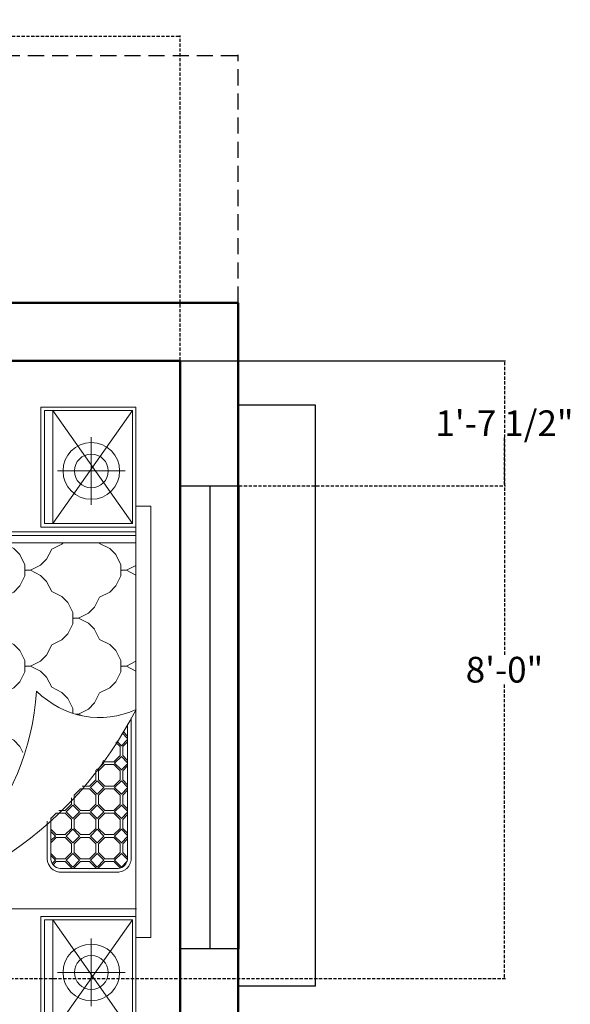
# Model space of a CAD drawing. Units: inches. Extents: x 513 to 1142, y 396 to 927.
# Tile 31 of 31: x 1056 to 1142, y 770 to 923. Entities that reach past the tile are written whole.
import ezdxf

# ---------------------------------------------------------------- set-up
doc = ezdxf.new("R2010")
doc.units = ezdxf.units.IN
doc.header["$MEASUREMENT"] = 0
doc.linetypes.add('DASHED', pattern=[0.75, 0.5, -0.25])
for name, color, linetype, lineweight in [('A-ANNO-DIMS', 2, 'DASHED', 18), ('A-WALL', 7, 'Continuous', 50), ('furniture', 92, 'Continuous', 18), ('windows', 172, 'Continuous', 25)]:
    doc.layers.add(name, color=color, linetype=linetype, lineweight=lineweight)
doc.styles.get("Standard").update_dxf_attribs({"font": 'arial.ttf'})
doc.dimstyles.get("Standard").update_dxf_attribs({"dimtxt": 4, "dimasz": 0.18, "dimexe": 0.18, "dimexo": 0.0625, "dimgap": 0.09, "dimtad": 0, "dimtih": 1, "dimtoh": 1, "dimdec": 0, "dimrnd": 6, "dimzin": 0, "dimdsep": 46, "dimlunit": 3, "dimtxsty": 'Standard', "dimcen": 0.09, "dimadec": 0, "dimazin": 0, "dimtfac": 1, "dimtdec": 0, "dimtofl": 0, "dimtmove": 0, "dimatfit": 3, "dimfxl": 1, "dimtolj": 1, "dimtzin": 0, "dimarcsym": 0})

# ---------------------------------------------------------------- blocks, each defined once
blk = doc.blocks.new('A$C029D5C69')
for p, q in [((0.4164, 2.0693), (0.4164, 2.0066)), ((2.2315, 2.0693), (0.4164, 2.0693)), ((2.2315, 2.0066), (2.2315, 2.0693)), ((0, 1.606), (0, 2.0066)), ((0, 2.0066), (0.505, 2.0066)), ((0.0151, 1.6211), (0.0151, 1.9915)), ((0.0151, 1.9915), (0.4899, 1.9915)), ((0.4164, 2.0066), (2.2315, 2.0066)), ((0.4899, 1.9915), (0.4899, 1.6211)), ((0.505, 2.0066), (0.505, 1.606)), ((0.5252, 0.0351), (0.5252, 2.0066)), ((0.5403, 0.0502), (0.5403, 2.0066)), ((0.5706, 0.0805), (0.5706, 2.0066)), ((0.6869, 1.966), (0.6666, 2.0066)), ((0.7072, 2.0066), (0.6869, 1.966)), ((1.0902, 1.966), (1.0699, 2.0066)), ((1.1106, 2.0066), (1.0902, 1.966)), ((2.1114, 2.0087), (2.1114, 0.0351)), ((2.6479, 2.0066), (2.1429, 2.0066)), ((2.1429, 2.0066), (2.1429, 1.606)), ((2.6328, 1.9915), (2.158, 1.9915)), ((2.158, 1.9915), (2.158, 1.6211)), ((2.6328, 1.6211), (2.6328, 1.9915)), ((2.6479, 1.606), (2.6479, 2.0066)), ((0.2689, 1.9609), (0.2689, 1.6764)), ((0.6869, 1.9425), (0.6869, 1.966)), ((0.6869, 1.9425), (0.6869, 1.966)), ((1.0902, 1.9425), (1.0902, 1.966)), ((1.0902, 1.9425), (1.0902, 1.966)), ((1.8954, 1.9865), (1.3081, 1.9865)), ((1.8954, 1.9713), (1.3339, 1.9713)), ((1.3849, 1.9713), (1.3656, 1.952)), ((1.3945, 1.9713), (1.3714, 1.9483)), ((1.4249, 1.945), (1.3986, 1.9713)), ((1.4288, 1.9507), (1.4081, 1.9713)), ((1.4476, 1.9507), (1.4288, 1.9507)), ((1.4476, 1.9507), (1.4664, 1.9507)), ((1.487, 1.9713), (1.4664, 1.9507)), ((1.4966, 1.9713), (1.4703, 1.945)), ((1.527, 1.945), (1.5007, 1.9713)), ((1.5309, 1.9507), (1.5102, 1.9713)), ((1.5497, 1.9507), (1.5309, 1.9507)), ((1.5497, 1.9507), (1.5685, 1.9507)), ((1.5891, 1.9713), (1.5685, 1.9507)), ((1.5987, 1.9713), (1.5724, 1.945)), ((1.6291, 1.945), (1.6028, 1.9713)), ((1.633, 1.9507), (1.6123, 1.9713)), ((1.6518, 1.9507), (1.633, 1.9507)), ((1.6518, 1.9507), (1.6706, 1.9507)), ((1.6912, 1.9713), (1.6706, 1.9507)), ((1.7008, 1.9713), (1.6745, 1.945)), ((1.7312, 1.945), (1.7049, 1.9713)), ((1.7351, 1.9507), (1.7144, 1.9713)), ((1.7539, 1.9507), (1.7351, 1.9507)), ((1.7539, 1.9507), (1.7727, 1.9507)), ((1.7933, 1.9713), (1.7727, 1.9507)), ((1.8029, 1.9713), (1.7766, 1.945)), ((1.8333, 1.945), (1.807, 1.9713)), ((1.8372, 1.9507), (1.8165, 1.9713)), ((1.856, 1.9507), (1.8372, 1.9507)), ((1.856, 1.9507), (1.8748, 1.9507)), ((1.8954, 1.9713), (1.8748, 1.9507)), ((1.9043, 1.9707), (1.8787, 1.945)), ((1.9354, 1.945), (1.9114, 1.969)), ((2.379, 1.9609), (2.379, 1.6764)), ((0.621, 1.9213), (0.5955, 1.8958)), ((0.6634, 1.9425), (0.621, 1.9213)), ((0.6634, 1.9425), (0.621, 1.9213)), ((0.6869, 1.9425), (0.6634, 1.9425)), ((0.6869, 1.9425), (0.7104, 1.9425)), ((0.7528, 1.9213), (0.7104, 1.9425)), ((0.7528, 1.9213), (0.7104, 1.9425)), ((0.7783, 1.8958), (0.7528, 1.9213)), ((1.0243, 1.9213), (0.9988, 1.8958)), ((1.0668, 1.9425), (1.0244, 1.9213)), ((1.0668, 1.9425), (1.0244, 1.9213)), ((1.0902, 1.9425), (1.0668, 1.9425)), ((1.0902, 1.9425), (1.1137, 1.9425)), ((1.1561, 1.9213), (1.1137, 1.9425)), ((1.1561, 1.9213), (1.1137, 1.9425)), ((1.1816, 1.8958), (1.1561, 1.9213)), ((1.4249, 1.945), (1.4059, 1.926)), ((1.4288, 1.9394), (1.4116, 1.9222)), ((1.4288, 1.9393), (1.4476, 1.9393)), ((1.4664, 1.9393), (1.4476, 1.9393)), ((1.493, 1.9128), (1.4664, 1.9394)), ((1.4986, 1.9167), (1.4703, 1.945)), ((1.493, 1.8752), (1.493, 1.9128)), ((1.527, 1.945), (1.4986, 1.9167)), ((1.5309, 1.9394), (1.5043, 1.9128)), ((1.5043, 1.8752), (1.5043, 1.9128)), ((1.5309, 1.9393), (1.5497, 1.9393)), ((1.5685, 1.9393), (1.5497, 1.9393)), ((1.595, 1.9128), (1.5685, 1.9394)), ((1.6007, 1.9167), (1.5724, 1.945)), ((1.595, 1.8752), (1.595, 1.9128)), ((1.6291, 1.945), (1.6007, 1.9167)), ((1.633, 1.9394), (1.6064, 1.9128)), ((1.6064, 1.8752), (1.6064, 1.9128)), ((1.633, 1.9393), (1.6518, 1.9393)), ((1.6706, 1.9393), (1.6518, 1.9393)), ((1.6971, 1.9128), (1.6706, 1.9394)), ((1.7028, 1.9167), (1.6745, 1.945)), ((1.6971, 1.8752), (1.6971, 1.9128)), ((1.7312, 1.945), (1.7028, 1.9167)), ((1.7351, 1.9394), (1.7085, 1.9128)), ((1.7085, 1.8752), (1.7085, 1.9128)), ((1.7351, 1.9393), (1.7539, 1.9393)), ((1.7727, 1.9393), (1.7539, 1.9393)), ((1.7992, 1.9128), (1.7727, 1.9394)), ((1.8049, 1.9167), (1.7766, 1.945)), ((1.7992, 1.8752), (1.7992, 1.9128)), ((1.8333, 1.945), (1.8049, 1.9167)), ((1.8372, 1.9394), (1.8106, 1.9128)), ((1.8106, 1.8752), (1.8106, 1.9128)), ((1.8372, 1.9393), (1.856, 1.9393)), ((1.8748, 1.9393), (1.856, 1.9393)), ((1.9013, 1.9128), (1.8748, 1.9394)), ((1.907, 1.9167), (1.8787, 1.945)), ((1.9013, 1.8752), (1.9013, 1.9128)), ((1.9354, 1.945), (1.907, 1.9167)), ((1.9393, 1.9394), (1.9127, 1.9128)), ((1.9127, 1.8752), (1.9127, 1.9128)), ((1.9393, 1.9393), (1.9404, 1.9393)), ((1.9414, 1.688), (1.9414, 1.931)), ((1.9565, 1.688), (1.9565, 1.931)), ((0.5955, 1.8958), (0.5743, 1.8534)), ((0.7995, 1.8534), (0.7783, 1.8958)), ((0.9989, 1.8958), (0.9777, 1.8534)), ((1.2028, 1.8534), (1.1816, 1.8958)), ((1.493, 1.8752), (1.4867, 1.869)), ((1.4986, 1.8713), (1.4922, 1.8648)), ((1.527, 1.8429), (1.4986, 1.8713)), ((1.5309, 1.8486), (1.5043, 1.8752)), ((1.595, 1.8752), (1.5685, 1.8486)), ((1.6007, 1.8713), (1.5724, 1.8429)), ((1.6291, 1.8429), (1.6007, 1.8713)), ((1.633, 1.8486), (1.6064, 1.8752)), ((1.6971, 1.8752), (1.6706, 1.8486)), ((1.7028, 1.8713), (1.6745, 1.8429)), ((1.7312, 1.8429), (1.7028, 1.8713)), ((1.7351, 1.8486), (1.7085, 1.8752)), ((1.7992, 1.8752), (1.7727, 1.8486)), ((1.8049, 1.8713), (1.7766, 1.8429)), ((1.8333, 1.8429), (1.8049, 1.8713)), ((1.8372, 1.8486), (1.8106, 1.8752)), ((1.9013, 1.8752), (1.8748, 1.8486)), ((1.907, 1.8713), (1.8787, 1.8429)), ((1.9354, 1.8429), (1.907, 1.8713)), ((1.9393, 1.8486), (1.9127, 1.8752)), ((0.5743, 1.8534), (0.5706, 1.8515)), ((0.5743, 1.8534), (0.5706, 1.8515)), ((0.8419, 1.8322), (0.7995, 1.8534)), ((0.8419, 1.8322), (0.7995, 1.8534)), ((0.8674, 1.8067), (0.8419, 1.8322)), ((0.9352, 1.8322), (0.9097, 1.8067)), ((0.9777, 1.8534), (0.9353, 1.8322)), ((0.9777, 1.8534), (0.9353, 1.8322)), ((1.2452, 1.8322), (1.2028, 1.8534)), ((1.2452, 1.8322), (1.2028, 1.8534)), ((1.2707, 1.8067), (1.2452, 1.8322)), ((1.527, 1.8429), (1.5242, 1.8401)), ((1.5309, 1.8373), (1.5295, 1.8359)), ((1.5497, 1.8486), (1.5309, 1.8486)), ((1.5309, 1.8373), (1.5497, 1.8373)), ((1.5497, 1.8486), (1.5685, 1.8486)), ((1.5685, 1.8373), (1.5497, 1.8373)), ((1.595, 1.8107), (1.5685, 1.8373)), ((1.6007, 1.8146), (1.5724, 1.8429)), ((1.6291, 1.8429), (1.6007, 1.8146)), ((1.633, 1.8373), (1.6064, 1.8107)), ((1.6518, 1.8486), (1.633, 1.8486)), ((1.633, 1.8373), (1.6518, 1.8373)), ((1.6518, 1.8486), (1.6706, 1.8486)), ((1.6706, 1.8373), (1.6518, 1.8373)), ((1.6971, 1.8107), (1.6706, 1.8373)), ((1.7028, 1.8146), (1.6745, 1.8429)), ((1.7312, 1.8429), (1.7028, 1.8146)), ((1.7351, 1.8373), (1.7085, 1.8107)), ((1.7539, 1.8486), (1.7351, 1.8486)), ((1.7351, 1.8373), (1.7539, 1.8373)), ((1.7539, 1.8486), (1.7727, 1.8486)), ((1.7727, 1.8373), (1.7539, 1.8373)), ((1.7992, 1.8107), (1.7727, 1.8373)), ((1.8049, 1.8146), (1.7766, 1.8429)), ((1.8333, 1.8429), (1.8049, 1.8146)), ((1.8372, 1.8373), (1.8106, 1.8107)), ((1.856, 1.8486), (1.8372, 1.8486)), ((1.8372, 1.8373), (1.856, 1.8373)), ((1.856, 1.8486), (1.8748, 1.8486)), ((1.8748, 1.8373), (1.856, 1.8373)), ((1.9013, 1.8107), (1.8748, 1.8373)), ((1.907, 1.8146), (1.8787, 1.8429)), ((1.9354, 1.8429), (1.907, 1.8146)), ((1.9393, 1.8373), (1.9127, 1.8107)), ((1.9414, 1.8486), (1.9393, 1.8486)), ((1.9393, 1.8373), (1.9414, 1.8373)), ((0.1267, 1.8186), (0.4111, 1.8186)), ((0.8886, 1.7643), (0.8674, 1.8067)), ((0.9098, 1.8067), (0.8886, 1.7643)), ((1.2919, 1.7643), (1.2707, 1.8067)), ((1.595, 1.7806), (1.595, 1.8107)), ((1.6064, 1.7731), (1.6064, 1.8107)), ((1.6971, 1.7731), (1.6971, 1.8107)), ((1.7085, 1.7731), (1.7085, 1.8107)), ((1.7992, 1.7731), (1.7992, 1.8107)), ((1.8106, 1.7731), (1.8106, 1.8107)), ((1.9013, 1.7731), (1.9013, 1.8107)), ((1.9127, 1.7731), (1.9127, 1.8107)), ((2.2367, 1.8186), (2.5212, 1.8186)), ((0.8651, 1.7408), (0.8227, 1.7196)), ((0.8651, 1.7408), (0.8227, 1.7196)), ((0.912, 1.7408), (0.8651, 1.7408)), ((0.8886, 1.7408), (0.8886, 1.7643)), ((0.9544, 1.7196), (0.912, 1.7408)), ((0.9544, 1.7196), (0.912, 1.7408)), ((1.2684, 1.7408), (1.226, 1.7196)), ((1.2684, 1.7408), (1.226, 1.7196)), ((1.2885, 1.7408), (1.2684, 1.7408)), ((1.2981, 1.7768), (1.2919, 1.7643)), ((1.2919, 1.7519), (1.2919, 1.7643)), ((1.633, 1.7465), (1.6064, 1.7731)), ((1.6518, 1.7465), (1.633, 1.7465)), ((1.6518, 1.7465), (1.6706, 1.7465)), ((1.6971, 1.7731), (1.6706, 1.7465)), ((1.7028, 1.7692), (1.6745, 1.7408)), ((1.7028, 1.7125), (1.6745, 1.7408)), ((1.7312, 1.7408), (1.7028, 1.7692)), ((1.7312, 1.7408), (1.7028, 1.7125)), ((1.7351, 1.7465), (1.7085, 1.7731)), ((1.7539, 1.7465), (1.7351, 1.7465)), ((1.7539, 1.7465), (1.7727, 1.7465)), ((1.7992, 1.7731), (1.7727, 1.7465)), ((1.8049, 1.7692), (1.7766, 1.7408)), ((1.8049, 1.7125), (1.7766, 1.7408)), ((1.8333, 1.7408), (1.8049, 1.7692)), ((1.8333, 1.7408), (1.8049, 1.7125)), ((1.8372, 1.7465), (1.8106, 1.7731)), ((1.856, 1.7465), (1.8372, 1.7465)), ((1.856, 1.7465), (1.8748, 1.7465)), ((1.9013, 1.7731), (1.8748, 1.7465)), ((1.907, 1.7692), (1.8787, 1.7408)), ((1.907, 1.7125), (1.8787, 1.7408)), ((1.9354, 1.7408), (1.907, 1.7692)), ((1.9354, 1.7408), (1.907, 1.7125)), ((1.9393, 1.7465), (1.9127, 1.7731)), ((1.9414, 1.7465), (1.9393, 1.7465)), ((0.5766, 1.6941), (0.5706, 1.7002)), ((0.8227, 1.7196), (0.7972, 1.6941)), ((0.98, 1.6941), (0.9545, 1.7196)), ((1.226, 1.7196), (1.2005, 1.6941)), ((1.6443, 1.7352), (1.6518, 1.7352)), ((1.6706, 1.7352), (1.6518, 1.7352)), ((1.6971, 1.7086), (1.6706, 1.7352)), ((1.6971, 1.682), (1.6971, 1.7086)), ((1.7351, 1.7352), (1.7085, 1.7086)), ((1.7085, 1.671), (1.7085, 1.7086)), ((1.7351, 1.7352), (1.7539, 1.7352)), ((1.7727, 1.7352), (1.7539, 1.7352)), ((1.7992, 1.7086), (1.7727, 1.7352)), ((1.7992, 1.671), (1.7992, 1.7086)), ((1.8372, 1.7352), (1.8106, 1.7086)), ((1.8106, 1.671), (1.8106, 1.7086)), ((1.8372, 1.7352), (1.856, 1.7352)), ((1.8748, 1.7352), (1.856, 1.7352)), ((1.9013, 1.7086), (1.8748, 1.7352)), ((1.9013, 1.671), (1.9013, 1.7086)), ((1.9393, 1.7352), (1.9127, 1.7086)), ((1.9127, 1.671), (1.9127, 1.7086)), ((1.9393, 1.7352), (1.9414, 1.7352)), ((0.5978, 1.6517), (0.5766, 1.6941)), ((0.7972, 1.6941), (0.776, 1.6517)), ((1.0011, 1.6517), (0.9799, 1.6941)), ((1.2005, 1.6941), (1.1793, 1.6517)), ((1.7318, 1.6477), (1.7085, 1.671)), ((1.7992, 1.671), (1.7759, 1.6477)), ((1.8049, 1.6671), (1.7855, 1.6477)), ((1.8244, 1.6477), (1.8049, 1.6671)), ((1.8339, 1.6477), (1.8106, 1.671)), ((1.9013, 1.671), (1.878, 1.6477)), ((1.907, 1.6671), (1.8876, 1.6477)), ((1.9202, 1.6539), (1.907, 1.6671)), ((1.926, 1.6577), (1.9127, 1.671)), ((2.5551, 1.6275), (2.5551, 1.696)), ((0.4899, 1.6211), (0.0151, 1.6211)), ((0.6402, 1.6305), (0.5978, 1.6517)), ((0.6402, 1.6305), (0.5978, 1.6517)), ((0.6657, 1.605), (0.6402, 1.6305)), ((0.7336, 1.6305), (0.7081, 1.605)), ((0.776, 1.6517), (0.7336, 1.6305)), ((0.776, 1.6517), (0.7336, 1.6305)), ((1.0435, 1.6305), (1.0011, 1.6517)), ((1.0435, 1.6305), (1.0011, 1.6517)), ((1.0691, 1.605), (1.0436, 1.6305)), ((1.1369, 1.6305), (1.1114, 1.605)), ((1.1793, 1.6517), (1.1369, 1.6305)), ((1.1793, 1.6517), (1.1369, 1.6305)), ((1.8961, 1.6477), (1.7289, 1.6477)), ((1.8961, 1.6325), (1.7422, 1.6325)), ((2.158, 1.6211), (2.6328, 1.6211)), ((0.505, 1.606), (0, 1.606)), ((0.6869, 1.5626), (0.6657, 1.605)), ((0.7081, 1.605), (0.6869, 1.5626)), ((1.0902, 1.5626), (1.069, 1.605)), ((1.1114, 1.605), (1.0902, 1.5626)), ((2.1429, 1.606), (2.6479, 1.606)), ((0.6634, 1.5391), (0.621, 1.5179)), ((0.6634, 1.5391), (0.621, 1.5179)), ((0.6869, 1.5392), (0.6634, 1.5392)), ((0.6869, 1.5392), (0.6869, 1.5626)), ((0.6869, 1.5392), (0.6869, 1.5626)), ((0.6869, 1.5392), (0.7104, 1.5392)), ((0.7528, 1.5179), (0.7104, 1.5391)), ((0.7528, 1.5179), (0.7104, 1.5391)), ((1.0668, 1.5391), (1.0244, 1.5179)), ((1.0668, 1.5391), (1.0244, 1.5179)), ((1.0902, 1.5392), (1.0668, 1.5392)), ((1.0902, 1.5392), (1.0902, 1.5626)), ((1.0902, 1.5392), (1.0902, 1.5626)), ((1.0902, 1.5392), (1.1137, 1.5392)), ((1.1561, 1.5179), (1.1137, 1.5391)), ((1.1561, 1.5179), (1.1137, 1.5391)), ((0.5955, 1.4925), (0.5743, 1.4501)), ((0.621, 1.5179), (0.5955, 1.4924)), ((0.7783, 1.4924), (0.7528, 1.5179)), ((0.7995, 1.4501), (0.7783, 1.4925)), ((0.9989, 1.4925), (0.9777, 1.4501)), ((1.0243, 1.5179), (0.9988, 1.4924)), ((1.1816, 1.4924), (1.1561, 1.5179)), ((1.2028, 1.4501), (1.1816, 1.4925)), ((1.4022, 1.4925), (1.381, 1.4501)), ((1.4277, 1.5179), (1.4022, 1.4924)), ((1.4534, 1.5308), (1.4277, 1.5179)), ((1.4534, 1.5308), (1.4277, 1.5179)), ((1.6062, 1.4501), (1.5966, 1.4692)), ((0.5403, 1.4117), (0.5706, 1.4117)), ((0.5743, 1.45), (0.5706, 1.4481)), ((0.5743, 1.45), (0.5706, 1.4481)), ((0.8419, 1.4288), (0.7995, 1.45)), ((0.8419, 1.4288), (0.7995, 1.45)), ((0.8674, 1.4033), (0.8419, 1.4288)), ((0.9352, 1.4288), (0.9097, 1.4033)), ((0.9777, 1.45), (0.9353, 1.4288)), ((0.9777, 1.45), (0.9353, 1.4288)), ((1.2452, 1.4288), (1.2028, 1.45)), ((1.2452, 1.4288), (1.2028, 1.45)), ((1.2707, 1.4033), (1.2452, 1.4288)), ((1.3386, 1.4288), (1.3131, 1.4033)), ((1.381, 1.45), (1.3386, 1.4288)), ((1.381, 1.45), (1.3386, 1.4288)), ((1.6486, 1.4288), (1.6062, 1.45)), ((1.6486, 1.4288), (1.6062, 1.45)), ((1.6741, 1.4033), (1.6486, 1.4288)), ((0.8886, 1.361), (0.8674, 1.4034)), ((0.9098, 1.4034), (0.8886, 1.361)), ((1.2919, 1.361), (1.2707, 1.4034)), ((1.3131, 1.4034), (1.2919, 1.361)), ((1.6953, 1.361), (1.6741, 1.4034)), ((1.714, 1.3984), (1.6953, 1.361)), ((0.8651, 1.3374), (0.8227, 1.3162)), ((0.8651, 1.3374), (0.8227, 1.3162)), ((0.912, 1.3375), (0.8651, 1.3375)), ((0.8886, 1.3375), (0.8886, 1.3609)), ((0.9544, 1.3162), (0.912, 1.3374)), ((0.9544, 1.3162), (0.912, 1.3374)), ((1.2684, 1.3374), (1.226, 1.3162)), ((1.2684, 1.3374), (1.226, 1.3162)), ((1.3154, 1.3375), (1.2684, 1.3375)), ((1.2919, 1.3375), (1.2919, 1.3609)), ((1.3578, 1.3162), (1.3154, 1.3374)), ((1.3578, 1.3162), (1.3154, 1.3374)), ((1.6718, 1.3374), (1.6294, 1.3162)), ((1.6718, 1.3374), (1.6294, 1.3162)), ((1.7187, 1.3375), (1.6718, 1.3375)), ((1.6953, 1.3375), (1.6953, 1.3609)), ((1.7611, 1.3162), (1.7187, 1.3374)), ((1.7611, 1.3162), (1.7187, 1.3374)), ((0.5766, 1.2908), (0.5706, 1.2968)), ((0.5978, 1.2484), (0.5766, 1.2908)), ((0.7972, 1.2908), (0.776, 1.2484)), ((0.8227, 1.3163), (0.7972, 1.2908)), ((0.98, 1.2908), (0.9545, 1.3163)), ((1.0011, 1.2484), (0.9799, 1.2908)), ((1.2005, 1.2908), (1.1793, 1.2484)), ((1.226, 1.3163), (1.2005, 1.2908)), ((1.3833, 1.2908), (1.3578, 1.3163)), ((1.4045, 1.2484), (1.3833, 1.2908)), ((1.6039, 1.2908), (1.5827, 1.2484)), ((1.6294, 1.3163), (1.6039, 1.2908)), ((1.7867, 1.2908), (1.7611, 1.3163)), ((1.8078, 1.2484), (1.7866, 1.2908)), ((0.6402, 1.2271), (0.5978, 1.2483)), ((0.6402, 1.2271), (0.5978, 1.2483)), ((0.776, 1.2483), (0.7336, 1.2271)), ((0.776, 1.2483), (0.7336, 1.2271)), ((1.0435, 1.2271), (1.0011, 1.2483)), ((1.0435, 1.2271), (1.0011, 1.2483)), ((1.1793, 1.2483), (1.1369, 1.2271)), ((1.1793, 1.2483), (1.1369, 1.2271)), ((1.4469, 1.2271), (1.4045, 1.2483)), ((1.4469, 1.2271), (1.4045, 1.2483)), ((1.5827, 1.2483), (1.5403, 1.2271)), ((1.5827, 1.2483), (1.5403, 1.2271)), ((1.8502, 1.2271), (1.8078, 1.2483)), ((1.8502, 1.2271), (1.8078, 1.2483)), ((0.5403, 1.21), (0.5706, 1.21)), ((0.6657, 1.2017), (0.6402, 1.2272)), ((0.6869, 1.1593), (0.6657, 1.2017)), ((0.7081, 1.2017), (0.6869, 1.1593)), ((0.7336, 1.2272), (0.7081, 1.2017)), ((1.0691, 1.2017), (1.0436, 1.2272)), ((1.0902, 1.1593), (1.069, 1.2017)), ((1.1114, 1.2017), (1.0902, 1.1593)), ((1.1369, 1.2272), (1.1114, 1.2017)), ((1.4724, 1.2017), (1.4469, 1.2272)), ((1.4936, 1.1593), (1.4724, 1.2017)), ((1.5148, 1.2017), (1.4936, 1.1593)), ((1.5403, 1.2272), (1.5148, 1.2017)), ((1.8758, 1.2017), (1.8503, 1.2272)), ((1.8969, 1.1593), (1.8757, 1.2017)), ((1.9181, 1.2017), (1.8969, 1.1593)), ((1.9215, 1.2051), (1.9181, 1.2017)), ((0.6634, 1.1358), (0.621, 1.1146)), ((0.6634, 1.1358), (0.621, 1.1146)), ((0.6869, 1.1358), (0.6634, 1.1358)), ((0.6869, 1.1358), (0.6869, 1.1593)), ((0.6869, 1.1358), (0.6869, 1.1593)), ((0.6869, 1.1358), (0.7104, 1.1358)), ((0.7528, 1.1146), (0.7104, 1.1358)), ((0.7528, 1.1146), (0.7104, 1.1358)), ((1.0668, 1.1358), (1.0244, 1.1146)), ((1.0668, 1.1358), (1.0244, 1.1146)), ((1.0902, 1.1358), (1.0668, 1.1358)), ((1.0902, 1.1358), (1.0902, 1.1593)), ((1.0902, 1.1358), (1.0902, 1.1593)), ((1.0902, 1.1358), (1.1137, 1.1358)), ((1.1561, 1.1146), (1.1137, 1.1358)), ((1.1561, 1.1146), (1.1137, 1.1358)), ((1.4701, 1.1358), (1.4277, 1.1146)), ((1.4701, 1.1358), (1.4277, 1.1146)), ((1.4936, 1.1358), (1.4701, 1.1358)), ((1.4936, 1.1358), (1.4936, 1.1593)), ((1.4936, 1.1358), (1.4936, 1.1593)), ((1.4936, 1.1358), (1.5171, 1.1358)), ((1.5595, 1.1146), (1.5171, 1.1358)), ((1.5595, 1.1146), (1.5171, 1.1358)), ((1.8735, 1.1358), (1.8311, 1.1146)), ((1.8735, 1.1358), (1.8311, 1.1146)), ((1.8969, 1.1358), (1.8735, 1.1358)), ((1.8969, 1.1358), (1.8969, 1.1593)), ((1.8969, 1.1358), (1.8969, 1.1593)), ((1.8969, 1.1358), (1.9204, 1.1358)), ((1.9628, 1.1146), (1.9204, 1.1358)), ((1.9628, 1.1146), (1.9204, 1.1358)), ((0.5955, 1.0891), (0.5743, 1.0467)), ((0.621, 1.1146), (0.5955, 1.0891)), ((0.7783, 1.0891), (0.7528, 1.1146)), ((0.7995, 1.0467), (0.7783, 1.0891)), ((0.9989, 1.0891), (0.9777, 1.0467)), ((1.0243, 1.1146), (0.9988, 1.0891)), ((1.1816, 1.0891), (1.1561, 1.1146)), ((1.2028, 1.0467), (1.1816, 1.0891)), ((1.4022, 1.0891), (1.381, 1.0467)), ((1.4277, 1.1146), (1.4022, 1.0891)), ((1.585, 1.0891), (1.5595, 1.1146)), ((1.6062, 1.0467), (1.585, 1.0891)), ((1.8056, 1.0891), (1.7844, 1.0467)), ((1.831, 1.1146), (1.8055, 1.0891)), ((1.9883, 1.0891), (1.9628, 1.1146)), ((2.0095, 1.0467), (1.9883, 1.0891)), ((0.5743, 1.0467), (0.5706, 1.0448)), ((0.5743, 1.0467), (0.5706, 1.0448)), ((0.8419, 1.0255), (0.7995, 1.0467)), ((0.8419, 1.0255), (0.7995, 1.0467)), ((0.9777, 1.0467), (0.9353, 1.0255)), ((0.9777, 1.0467), (0.9353, 1.0255)), ((1.2452, 1.0255), (1.2028, 1.0467)), ((1.2452, 1.0255), (1.2028, 1.0467)), ((1.381, 1.0467), (1.3386, 1.0255)), ((1.381, 1.0467), (1.3386, 1.0255)), ((1.6486, 1.0255), (1.6062, 1.0467)), ((1.6486, 1.0255), (1.6062, 1.0467)), ((1.7844, 1.0467), (1.742, 1.0255)), ((1.7844, 1.0467), (1.742, 1.0255)), ((2.0276, 1.0376), (2.0095, 1.0467)), ((2.0276, 1.0376), (2.0095, 1.0467)), ((0.8674, 1), (0.8419, 1.0255)), ((0.8886, 0.9576), (0.8674, 1)), ((0.9098, 1), (0.8886, 0.9576)), ((0.9352, 1.0255), (0.9097, 1)), ((1.2707, 1), (1.2452, 1.0255)), ((1.2919, 0.9576), (1.2707, 1)), ((1.3131, 1), (1.2919, 0.9576)), ((1.3386, 1.0255), (1.3131, 1)), ((1.6741, 1), (1.6486, 1.0255)), ((1.6953, 0.9576), (1.6741, 1)), ((1.7165, 1), (1.6953, 0.9576)), ((1.7419, 1.0255), (1.7164, 1)), ((0.8886, 0.9341), (0.8886, 0.9576)), ((1.2919, 0.9341), (1.2919, 0.9576)), ((1.6953, 0.9341), (1.6953, 0.9576)), ((0.8227, 0.9129), (0.7972, 0.8874)), ((0.8651, 0.9341), (0.8227, 0.9129)), ((0.8651, 0.9341), (0.8227, 0.9129)), ((0.912, 0.9341), (0.8651, 0.9341)), ((0.9544, 0.9129), (0.912, 0.9341)), ((0.9544, 0.9129), (0.912, 0.9341)), ((0.98, 0.8874), (0.9545, 0.9129)), ((1.226, 0.9129), (1.2005, 0.8874)), ((1.2684, 0.9341), (1.226, 0.9129)), ((1.2684, 0.9341), (1.226, 0.9129)), ((1.3154, 0.9341), (1.2684, 0.9341)), ((1.3578, 0.9129), (1.3154, 0.9341)), ((1.3578, 0.9129), (1.3154, 0.9341)), ((1.3833, 0.8874), (1.3578, 0.9129)), ((1.6294, 0.9129), (1.6039, 0.8874)), ((1.6718, 0.9341), (1.6294, 0.9129)), ((1.6718, 0.9341), (1.6294, 0.9129)), ((1.7187, 0.9341), (1.6718, 0.9341)), ((1.7611, 0.9129), (1.7187, 0.9341)), ((1.7611, 0.9129), (1.7187, 0.9341)), ((1.7867, 0.8874), (1.7611, 0.9129)), ((2.0327, 0.9129), (2.0072, 0.8874)), ((2.066, 0.9295), (2.0327, 0.9129)), ((2.066, 0.9295), (2.0327, 0.9129)), ((2.066, 0.9457), (2.066, 0.0805)), ((0.5766, 0.8874), (0.5706, 0.8935)), ((0.5978, 0.845), (0.5766, 0.8874)), ((0.7972, 0.8874), (0.776, 0.845)), ((1.0011, 0.845), (0.9799, 0.8874)), ((1.2005, 0.8874), (1.1793, 0.845)), ((1.4045, 0.845), (1.3833, 0.8874)), ((1.6039, 0.8874), (1.5827, 0.845)), ((1.8078, 0.845), (1.7866, 0.8874)), ((2.0072, 0.8874), (1.986, 0.845)), ((0.6402, 0.8238), (0.5978, 0.845)), ((0.6402, 0.8238), (0.5978, 0.845)), ((0.776, 0.845), (0.7336, 0.8238)), ((0.776, 0.845), (0.7336, 0.8238)), ((1.0435, 0.8238), (1.0011, 0.845)), ((1.0435, 0.8238), (1.0011, 0.845)), ((1.1793, 0.845), (1.1369, 0.8238)), ((1.1793, 0.845), (1.1369, 0.8238)), ((1.4469, 0.8238), (1.4045, 0.845)), ((1.4469, 0.8238), (1.4045, 0.845)), ((1.5827, 0.845), (1.5403, 0.8238)), ((1.5827, 0.845), (1.5403, 0.8238)), ((1.8502, 0.8238), (1.8078, 0.845)), ((1.8502, 0.8238), (1.8078, 0.845)), ((1.986, 0.845), (1.9436, 0.8238)), ((1.986, 0.845), (1.9436, 0.8238)), ((2.0962, 0.8369), (2.0962, 0.0502)), ((0.6657, 0.7983), (0.6402, 0.8238)), ((0.6869, 0.7559), (0.6657, 0.7983)), ((0.7081, 0.7983), (0.6869, 0.7559)), ((0.7336, 0.8238), (0.7081, 0.7983)), ((1.0691, 0.7983), (1.0436, 0.8238)), ((1.0902, 0.7559), (1.069, 0.7983)), ((1.1114, 0.7983), (1.0902, 0.7559)), ((1.1369, 0.8238), (1.1114, 0.7983)), ((1.4724, 0.7983), (1.4469, 0.8238)), ((1.4936, 0.7559), (1.4724, 0.7983)), ((1.5148, 0.7983), (1.4936, 0.7559)), ((1.5403, 0.8238), (1.5148, 0.7983)), ((1.8758, 0.7983), (1.8503, 0.8238)), ((1.8969, 0.7559), (1.8757, 0.7983)), ((1.9181, 0.7983), (1.8969, 0.7559)), ((1.9436, 0.8238), (1.9181, 0.7983)), ((0.6869, 0.7325), (0.6869, 0.7559)), ((0.6869, 0.7325), (0.6869, 0.7559)), ((1.0902, 0.7325), (1.0902, 0.7559)), ((1.0902, 0.7325), (1.0902, 0.7559)), ((1.2024, 0.7028), (1.2503, 0.7507)), ((1.4936, 0.7325), (1.4936, 0.7559)), ((1.4936, 0.7325), (1.4936, 0.7559)), ((1.8969, 0.7325), (1.8969, 0.7559)), ((1.8969, 0.7325), (1.8969, 0.7559)), ((0.621, 0.7113), (0.5955, 0.6858)), ((0.6634, 0.7324), (0.621, 0.7112)), ((0.6634, 0.7324), (0.621, 0.7112)), ((0.6869, 0.7325), (0.6634, 0.7325)), ((0.6869, 0.7325), (0.7104, 0.7325)), ((0.7528, 0.7112), (0.7104, 0.7324)), ((0.7528, 0.7112), (0.7104, 0.7324)), ((0.7783, 0.6858), (0.7528, 0.7113)), ((1.0243, 0.7113), (0.9988, 0.6858)), ((1.0668, 0.7324), (1.0244, 0.7112)), ((1.0668, 0.7324), (1.0244, 0.7112)), ((1.0902, 0.7325), (1.0668, 0.7325)), ((1.0902, 0.7325), (1.1137, 0.7325)), ((1.1561, 0.7112), (1.1137, 0.7324)), ((1.1561, 0.7112), (1.1137, 0.7324)), ((1.1816, 0.6858), (1.1561, 0.7113)), ((1.4277, 0.7113), (1.4022, 0.6858)), ((1.4701, 0.7324), (1.4277, 0.7112)), ((1.4701, 0.7324), (1.4277, 0.7112)), ((1.4936, 0.7325), (1.4701, 0.7325)), ((1.4936, 0.7325), (1.5171, 0.7325)), ((1.5595, 0.7112), (1.5171, 0.7324)), ((1.5595, 0.7112), (1.5171, 0.7324)), ((1.585, 0.6858), (1.5595, 0.7113)), ((1.831, 0.7113), (1.8055, 0.6858)), ((1.8735, 0.7324), (1.8311, 0.7112)), ((1.8735, 0.7324), (1.8311, 0.7112)), ((1.8969, 0.7325), (1.8735, 0.7325)), ((1.8969, 0.7325), (1.9204, 0.7325)), ((1.9628, 0.7112), (1.9204, 0.7324)), ((1.9628, 0.7112), (1.9204, 0.7324)), ((1.9883, 0.6858), (1.9628, 0.7113)), ((0.5955, 0.6858), (0.5743, 0.6434)), ((0.7995, 0.6434), (0.7783, 0.6858)), ((0.9989, 0.6858), (0.9777, 0.6434)), ((1.2028, 0.6434), (1.1816, 0.6858)), ((1.4022, 0.6858), (1.381, 0.6434)), ((1.6062, 0.6434), (1.585, 0.6858)), ((1.8056, 0.6858), (1.7844, 0.6434)), ((2.0095, 0.6434), (1.9883, 0.6858)), ((0.5743, 0.6433), (0.5706, 0.6414)), ((0.5743, 0.6433), (0.5706, 0.6414)), ((0.8419, 0.6221), (0.7995, 0.6433)), ((0.8419, 0.6221), (0.7995, 0.6433)), ((0.8674, 0.5967), (0.8419, 0.6222)), ((0.9352, 0.6222), (0.9097, 0.5967)), ((0.9777, 0.6433), (0.9353, 0.6221)), ((0.9777, 0.6433), (0.9353, 0.6221)), ((1.2452, 0.6221), (1.2028, 0.6433)), ((1.2452, 0.6221), (1.2028, 0.6433)), ((1.2707, 0.5967), (1.2452, 0.6222)), ((1.3386, 0.6222), (1.3131, 0.5967)), ((1.381, 0.6433), (1.3386, 0.6221)), ((1.381, 0.6433), (1.3386, 0.6221)), ((1.6486, 0.6221), (1.6062, 0.6433)), ((1.6486, 0.6221), (1.6062, 0.6433)), ((1.6741, 0.5967), (1.6486, 0.6222)), ((1.7419, 0.6222), (1.7164, 0.5967)), ((1.7844, 0.6433), (1.742, 0.6221)), ((1.7844, 0.6433), (1.742, 0.6221)), ((2.0519, 0.6221), (2.0095, 0.6433)), ((2.0519, 0.6221), (2.0095, 0.6433)), ((2.066, 0.6081), (2.0519, 0.6222)), ((0.8886, 0.5543), (0.8674, 0.5967)), ((0.9098, 0.5967), (0.8886, 0.5543)), ((1.2919, 0.5543), (1.2707, 0.5967)), ((1.3131, 0.5967), (1.2919, 0.5543)), ((1.6953, 0.5543), (1.6741, 0.5967)), ((1.7165, 0.5967), (1.6953, 0.5543)), ((0.8886, 0.5308), (0.8886, 0.5543)), ((1.2919, 0.5308), (1.2919, 0.5543)), ((1.6953, 0.5308), (1.6953, 0.5543)), ((0.8227, 0.5096), (0.7972, 0.4841)), ((0.8651, 0.5308), (0.8227, 0.5096)), ((0.8651, 0.5308), (0.8227, 0.5096)), ((0.912, 0.5308), (0.8651, 0.5308)), ((0.9544, 0.5096), (0.912, 0.5308)), ((0.9544, 0.5096), (0.912, 0.5308)), ((0.98, 0.4841), (0.9545, 0.5096)), ((1.226, 0.5096), (1.2005, 0.4841)), ((1.2684, 0.5308), (1.226, 0.5096)), ((1.2684, 0.5308), (1.226, 0.5096)), ((1.3154, 0.5308), (1.2684, 0.5308)), ((1.3578, 0.5096), (1.3154, 0.5308)), ((1.3578, 0.5096), (1.3154, 0.5308)), ((1.3833, 0.4841), (1.3578, 0.5096)), ((1.6294, 0.5096), (1.6039, 0.4841)), ((1.6718, 0.5308), (1.6294, 0.5096)), ((1.6718, 0.5308), (1.6294, 0.5096)), ((1.7187, 0.5308), (1.6718, 0.5308)), ((1.7611, 0.5096), (1.7187, 0.5308)), ((1.7611, 0.5096), (1.7187, 0.5308)), ((1.7867, 0.4841), (1.7611, 0.5096)), ((2.0327, 0.5096), (2.0072, 0.4841)), ((2.066, 0.5262), (2.0327, 0.5096)), ((2.066, 0.5262), (2.0327, 0.5096)), ((0.5766, 0.4841), (0.5706, 0.4901)), ((0.5978, 0.4417), (0.5766, 0.4841)), ((0.7972, 0.4841), (0.776, 0.4417)), ((1.0011, 0.4417), (0.9799, 0.4841)), ((1.2005, 0.4841), (1.1793, 0.4417)), ((1.4045, 0.4417), (1.3833, 0.4841)), ((1.6039, 0.4841), (1.5827, 0.4417)), ((1.8078, 0.4417), (1.7866, 0.4841)), ((2.0072, 0.4841), (1.986, 0.4417)), ((0.6402, 0.4205), (0.5978, 0.4417)), ((0.6402, 0.4205), (0.5978, 0.4417)), ((0.6657, 0.395), (0.6402, 0.4205)), ((0.7336, 0.4205), (0.7081, 0.395)), ((0.776, 0.4417), (0.7336, 0.4205)), ((0.776, 0.4417), (0.7336, 0.4205)), ((1.0435, 0.4205), (1.0011, 0.4417)), ((1.0435, 0.4205), (1.0011, 0.4417)), ((1.0691, 0.395), (1.0436, 0.4205)), ((1.1369, 0.4205), (1.1114, 0.395)), ((1.1793, 0.4417), (1.1369, 0.4205)), ((1.1793, 0.4417), (1.1369, 0.4205)), ((1.4469, 0.4205), (1.4045, 0.4417)), ((1.4469, 0.4205), (1.4045, 0.4417)), ((1.4724, 0.395), (1.4469, 0.4205)), ((1.5403, 0.4205), (1.5148, 0.395)), ((1.5827, 0.4417), (1.5403, 0.4205)), ((1.5827, 0.4417), (1.5403, 0.4205)), ((1.8502, 0.4205), (1.8078, 0.4417)), ((1.8502, 0.4205), (1.8078, 0.4417)), ((1.8758, 0.395), (1.8503, 0.4205)), ((1.9436, 0.4205), (1.9181, 0.395)), ((1.986, 0.4417), (1.9436, 0.4205)), ((1.986, 0.4417), (1.9436, 0.4205)), ((0.6869, 0.3526), (0.6657, 0.395)), ((0.7081, 0.395), (0.6869, 0.3526)), ((1.0902, 0.3526), (1.069, 0.395)), ((1.1114, 0.395), (1.0902, 0.3526)), ((1.4936, 0.3526), (1.4724, 0.395)), ((1.5148, 0.395), (1.4936, 0.3526)), ((1.8969, 0.3526), (1.8757, 0.395)), ((1.9181, 0.395), (1.8969, 0.3526)), ((0.6869, 0.3291), (0.6869, 0.3526)), ((0.6869, 0.3291), (0.6869, 0.3526)), ((1.0902, 0.3291), (1.0902, 0.3526)), ((1.0902, 0.3291), (1.0902, 0.3526)), ((1.4936, 0.3291), (1.4936, 0.3526)), ((1.4936, 0.3291), (1.4936, 0.3526)), ((1.8969, 0.3291), (1.8969, 0.3526)), ((1.8969, 0.3291), (1.8969, 0.3526)), ((0.621, 0.3079), (0.5955, 0.2824)), ((0.6634, 0.3291), (0.621, 0.3079)), ((0.6634, 0.3291), (0.621, 0.3079)), ((0.6869, 0.3291), (0.6634, 0.3291)), ((0.6869, 0.3291), (0.7104, 0.3291)), ((0.7528, 0.3079), (0.7104, 0.3291)), ((0.7528, 0.3079), (0.7104, 0.3291)), ((0.7783, 0.2824), (0.7528, 0.3079)), ((1.0243, 0.3079), (0.9988, 0.2824)), ((1.0668, 0.3291), (1.0244, 0.3079)), ((1.0668, 0.3291), (1.0244, 0.3079)), ((1.0902, 0.3291), (1.0668, 0.3291)), ((1.0902, 0.3291), (1.1137, 0.3291)), ((1.1561, 0.3079), (1.1137, 0.3291)), ((1.1561, 0.3079), (1.1137, 0.3291)), ((1.1816, 0.2824), (1.1561, 0.3079)), ((1.4277, 0.3079), (1.4022, 0.2824)), ((1.4701, 0.3291), (1.4277, 0.3079)), ((1.4701, 0.3291), (1.4277, 0.3079)), ((1.4936, 0.3291), (1.4701, 0.3291)), ((1.4936, 0.3291), (1.5171, 0.3291)), ((1.5595, 0.3079), (1.5171, 0.3291)), ((1.5595, 0.3079), (1.5171, 0.3291)), ((1.585, 0.2824), (1.5595, 0.3079)), ((1.831, 0.3079), (1.8055, 0.2824)), ((1.8735, 0.3291), (1.8311, 0.3079)), ((1.8735, 0.3291), (1.8311, 0.3079)), ((1.8969, 0.3291), (1.8735, 0.3291)), ((1.8969, 0.3291), (1.9204, 0.3291)), ((1.9628, 0.3079), (1.9204, 0.3291)), ((1.9628, 0.3079), (1.9204, 0.3291)), ((1.9883, 0.2824), (1.9628, 0.3079)), ((0.5955, 0.2824), (0.5743, 0.24)), ((0.7995, 0.24), (0.7783, 0.2824)), ((0.9989, 0.2824), (0.9777, 0.24)), ((1.2028, 0.24), (1.1816, 0.2824)), ((1.4022, 0.2824), (1.381, 0.24)), ((1.6062, 0.24), (1.585, 0.2824)), ((1.8056, 0.2824), (1.7844, 0.24)), ((2.0095, 0.24), (1.9883, 0.2824)), ((0.5743, 0.24), (0.5706, 0.2381)), ((0.5743, 0.24), (0.5706, 0.2381)), ((0.8419, 0.2188), (0.7995, 0.24)), ((0.8419, 0.2188), (0.7995, 0.24)), ((0.8674, 0.1933), (0.8419, 0.2188)), ((0.9352, 0.2188), (0.9097, 0.1933)), ((0.9777, 0.24), (0.9353, 0.2188)), ((0.9777, 0.24), (0.9353, 0.2188)), ((1.2452, 0.2188), (1.2028, 0.24)), ((1.2452, 0.2188), (1.2028, 0.24)), ((1.2707, 0.1933), (1.2452, 0.2188)), ((1.3386, 0.2188), (1.3131, 0.1933)), ((1.381, 0.24), (1.3386, 0.2188)), ((1.381, 0.24), (1.3386, 0.2188)), ((1.6486, 0.2188), (1.6062, 0.24)), ((1.6486, 0.2188), (1.6062, 0.24)), ((1.6741, 0.1933), (1.6486, 0.2188)), ((1.7419, 0.2188), (1.7164, 0.1933)), ((1.7844, 0.24), (1.742, 0.2188)), ((1.7844, 0.24), (1.742, 0.2188)), ((2.0519, 0.2188), (2.0095, 0.24)), ((2.0519, 0.2188), (2.0095, 0.24)), ((2.066, 0.2047), (2.0519, 0.2188)), ((0.8886, 0.1509), (0.8674, 0.1933)), ((0.9098, 0.1933), (0.8886, 0.1509)), ((1.2919, 0.1509), (1.2707, 0.1933)), ((1.3131, 0.1933), (1.2919, 0.1509)), ((1.6953, 0.1509), (1.6741, 0.1933)), ((1.7165, 0.1933), (1.6953, 0.1509)), ((0.8651, 0.1274), (0.8227, 0.1062)), ((0.8651, 0.1274), (0.8227, 0.1062)), ((0.912, 0.1275), (0.8651, 0.1275)), ((0.8886, 0.1275), (0.8886, 0.1509)), ((0.9544, 0.1062), (0.912, 0.1274)), ((0.9544, 0.1062), (0.912, 0.1274)), ((1.2684, 0.1274), (1.226, 0.1062)), ((1.2684, 0.1274), (1.226, 0.1062)), ((1.3154, 0.1275), (1.2684, 0.1275)), ((1.2919, 0.1275), (1.2919, 0.1509)), ((1.3578, 0.1062), (1.3154, 0.1274)), ((1.3578, 0.1062), (1.3154, 0.1274)), ((1.6718, 0.1274), (1.6294, 0.1062)), ((1.6718, 0.1274), (1.6294, 0.1062)), ((1.7187, 0.1275), (1.6718, 0.1275)), ((1.6953, 0.1275), (1.6953, 0.1509)), ((1.7611, 0.1062), (1.7187, 0.1274)), ((1.7611, 0.1062), (1.7187, 0.1274)), ((0.5766, 0.0807), (0.5706, 0.0868)), ((0.8227, 0.1062), (0.7972, 0.0807)), ((0.98, 0.0807), (0.9545, 0.1062)), ((1.226, 0.1062), (1.2005, 0.0807)), ((1.3833, 0.0807), (1.3578, 0.1062)), ((1.6294, 0.1062), (1.6039, 0.0807)), ((1.7867, 0.0807), (1.7611, 0.1062)), ((2.0327, 0.1062), (2.0072, 0.0807)), ((2.066, 0.1228), (2.0327, 0.1062)), ((2.066, 0.1228), (2.0327, 0.1062)), ((0.5978, 0.0384), (0.5766, 0.0808)), ((2.0309, 0.0454), (0.6056, 0.0454)), ((0.7972, 0.0808), (0.776, 0.0384)), ((1.0011, 0.0384), (0.9799, 0.0808)), ((1.2005, 0.0808), (1.1793, 0.0384)), ((1.4045, 0.0384), (1.3833, 0.0808)), ((1.6039, 0.0808), (1.5827, 0.0384)), ((1.8078, 0.0384), (1.7866, 0.0808)), ((2.0072, 0.0808), (1.986, 0.0384)), ((2.0763, 0), (0.5603, 0)), ((2.0612, 0.0151), (0.5754, 0.0151)), ((0.6402, 0.0171), (0.5978, 0.0383)), ((0.6402, 0.0171), (0.5978, 0.0383)), ((0.6523, 0.005), (0.6402, 0.0171)), ((0.7336, 0.0171), (0.7215, 0.005)), ((0.776, 0.0383), (0.7336, 0.0171)), ((0.776, 0.0383), (0.7336, 0.0171)), ((1.0435, 0.0171), (1.0011, 0.0383)), ((1.0435, 0.0171), (1.0011, 0.0383)), ((1.0557, 0.005), (1.0436, 0.0171)), ((1.1369, 0.0171), (1.1248, 0.005)), ((1.1793, 0.0383), (1.1369, 0.0171)), ((1.1793, 0.0383), (1.1369, 0.0171)), ((1.4469, 0.0171), (1.4045, 0.0383)), ((1.4469, 0.0171), (1.4045, 0.0383)), ((1.459, 0.005), (1.4469, 0.0171)), ((1.5403, 0.0171), (1.5282, 0.005)), ((1.5827, 0.0383), (1.5403, 0.0171)), ((1.5827, 0.0383), (1.5403, 0.0171)), ((1.8502, 0.0171), (1.8078, 0.0383)), ((1.8502, 0.0171), (1.8078, 0.0383)), ((1.8623, 0.005), (1.8503, 0.0171)), ((1.9436, 0.0171), (1.9315, 0.005)), ((1.986, 0.0383), (1.9436, 0.0171)), ((1.986, 0.0383), (1.9436, 0.0171))]:
    blk.add_line(p, q)
at = {"ltscale": 0.005}
for p, q in [((0.4899, 1.6568), (0.0151, 1.9915)), ((0.0151, 1.6568), (0.4899, 1.9915)), ((2.6328, 1.6568), (2.158, 1.9915)), ((2.158, 1.6568), (2.6328, 1.9915)), ((0.0151, 1.6568), (0.4899, 1.6568)), ((2.6328, 1.6568), (2.158, 1.6568))]:
    blk.add_line(p, q, dxfattribs=at)
for centre, radius in [((0.2689, 1.8186), 0.1191), ((2.379, 1.8186), 0.1191), ((0.2689, 1.8186), 0.0711), ((2.379, 1.8186), 0.0711)]:
    blk.add_circle(centre, radius)
for centre, radius, start, end in [((0.2843, 0.0157), 0.6251, 10.2961, 13.2684), ((0.5754, 0.0502), 0.0351, 180, 270), ((0.6056, 0.0805), 0.0351, 180, 270), ((2.0309, 0.0805), 0.0351, 270, 0), ((2.0612, 0.0502), 0.0351, 270, 0), ((0.5603, 0.0351), 0.0351, 180, 270), ((2.0763, 0.0351), 0.0351, 270, 0)]:
    blk.add_arc(centre, radius, start, end)
for centre, major_axis, ratio, start_param, end_param in [((0.8506, 1.8527), (-0.4556, 0), 0.89, 2.430919, 3.53111), ((0.3667, 0.6698), (1.7398, 0.1668), 0.88072, -0.045073, 0.941433), ((1.8961, 1.931), (-0.0453, 0), 0.89, 3.141593, 4.712389), ((1.8961, 1.688), (-0.0453, 0), 0.89, 1.570796, 3.141593), ((1.0874, 0.6748), (1.021, 0.1213), 0.889348, -0.031673, 1.359628)]:
    blk.add_ellipse(centre, major_axis=major_axis, ratio=ratio, start_param=start_param, end_param=end_param)
for points, knots in [([(1.9565, 1.931), (1.9565, 1.9336), (1.9563, 1.9362), (1.9553, 1.9428), (1.9543, 1.9467), (1.9512, 1.9541), (1.9493, 1.9577), (1.9446, 1.9643), (1.942, 1.9674), (1.936, 1.9729), (1.9327, 1.9753), (1.9257, 1.9795), (1.922, 1.9813), (1.9142, 1.9841), (1.9102, 1.9851), (1.9028, 1.9862), (1.8995, 1.9865), (1.8961, 1.9865)], [3.141593, 3.141593, 3.141593, 3.141593, 3.277614, 3.277614, 3.488082, 3.488082, 3.698551, 3.698551, 3.909019, 3.909019, 4.119488, 4.119488, 4.329956, 4.329956, 4.540424, 4.540424, 4.712389, 4.712389, 4.712389, 4.712389]), ([(1.8961, 1.6325), (1.899, 1.6325), (1.9019, 1.6327), (1.9101, 1.6338), (1.9153, 1.6352), (1.9253, 1.6392), (1.93, 1.6418), (1.9385, 1.6481), (1.9423, 1.6519), (1.9481, 1.6594), (1.9503, 1.663), (1.9537, 1.6707), (1.955, 1.6747), (1.9563, 1.6818), (1.9565, 1.6849), (1.9565, 1.688)], [1.570796, 1.570796, 1.570796, 1.570796, 1.718836, 1.718836, 1.993452, 1.993452, 2.268068, 2.268068, 2.542684, 2.542684, 2.761386, 2.761386, 2.980087, 2.980087, 3.141593, 3.141593, 3.141593, 3.141593])]:
    blk.add_open_spline(points, degree=3, knots=knots)
blk = doc.blocks.new('A$C0D3A6DFA')
blk.add_blockref('A$C029D5C69', (0, 0))
blk = doc.blocks.new('*D103')
at = {"layer": 'A-ANNO-DIMS', "color": 0, "lineweight": -2, "ltscale": 5, "transparency": 16777216}
for p, q in [((575, 879.22), (575, 917.74)), ((575.18, 917.56), (828.93, 917.56)), ((1089.82, 917.56), (836.06, 917.56)), ((1090, 879.22), (1090, 917.74))]:
    blk.add_line(p, q, dxfattribs=at)
at = {"layer": 'A-ANNO-DIMS', "color": 0, "ltscale": 5, "transparency": 16777216}
for points in [[(575.18, 917.59), (575.18, 917.53), (575, 917.56)], [(1089.82, 917.59), (1089.82, 917.53), (1090, 917.56)]]:
    blk.add_solid(points, dxfattribs=at)
at = {"layer": 'Defpoints', "color": 0, "ltscale": 5, "transparency": 16777216}
for p in [(1090, 917.56), (575, 879.16), (1090, 879.16)]:
    blk.add_point(p, dxfattribs=at)
at = {"layer": 'A-ANNO-DIMS', "color": 0, "ltscale": 5, "transparency": 16777216, "insert": (832.5, 917.56), "char_height": 4, "attachment_point": 5}
blk.add_mtext("\\A1;43'", dxfattribs=at)
blk = doc.blocks.new('WIN-72IN')
blk.add_line((0, 4.45), (72, 4.45))
blk.add_lwpolyline([(72, 9), (72, 0), (0, 0), (0, 9)], close=True)
blk = doc.blocks.new('*D138')
at = {"layer": 'A-ANNO-DIMS', "color": 0, "lineweight": -2, "transparency": 16777216}
for p, q in [((925, 870.22), (925, 920.74)), ((925.18, 920.56), (996.22, 920.56)), ((1080.82, 920.56), (1009.77, 920.56)), ((1081, 870.22), (1081, 920.74))]:
    blk.add_line(p, q, dxfattribs=at)
at = {"layer": 'A-ANNO-DIMS', "color": 0, "transparency": 16777216}
for points in [[(925.18, 920.59), (925.18, 920.53), (925, 920.56)], [(1080.82, 920.59), (1080.82, 920.53), (1081, 920.56)]]:
    blk.add_solid(points, dxfattribs=at)
at = {"layer": 'Defpoints', "color": 0, "transparency": 16777216}
for p in [(1081, 920.56), (925, 870.16), (1081, 870.16)]:
    blk.add_point(p, dxfattribs=at)
at = {"layer": 'A-ANNO-DIMS', "color": 0, "transparency": 16777216, "insert": (1003, 920.56), "char_height": 4, "attachment_point": 5}
blk.add_mtext('\\A1;13\'-0"', dxfattribs=at)
blk = doc.blocks.new('*D148')
at = {"layer": 'A-ANNO-DIMS', "color": 0, "lineweight": -2, "transparency": 16777216}
for p, q in [((921.06, 870.16), (1131.58, 870.16)), ((1131.4, 869.98), (1131.4, 824.29)), ((1131.4, 774.34), (1131.4, 820.03)), ((897.06, 774.16), (1131.58, 774.16))]:
    blk.add_line(p, q, dxfattribs=at)
at = {"layer": 'A-ANNO-DIMS', "color": 0, "transparency": 16777216}
for points in [[(1131.37, 869.98), (1131.43, 869.98), (1131.4, 870.16)], [(1131.37, 774.34), (1131.43, 774.34), (1131.4, 774.16)]]:
    blk.add_solid(points, dxfattribs=at)
at = {"layer": 'Defpoints', "color": 0, "transparency": 16777216}
for p in [(921, 870.16), (1131.4, 870.16), (897, 774.16)]:
    blk.add_point(p, dxfattribs=at)
at = {"layer": 'A-ANNO-DIMS', "color": 0, "transparency": 16777216, "insert": (1131.4, 822.16), "char_height": 4, "attachment_point": 5}
blk.add_mtext('\\A1;8\'-0"', dxfattribs=at)
blk = doc.blocks.new('*D161')
at = {"layer": 'A-ANNO-DIMS', "color": 0, "lineweight": -2, "transparency": 16777216}
for p, q in [((1081.06, 870.16), (1131.58, 870.16)), ((1131.4, 869.98), (1131.4, 862.62)), ((1131.4, 850.94), (1131.4, 858.3)), ((1081.14, 850.76), (1131.58, 850.76))]:
    blk.add_line(p, q, dxfattribs=at)
at = {"layer": 'A-ANNO-DIMS', "color": 0, "transparency": 16777216}
for points in [[(1131.37, 869.98), (1131.43, 869.98), (1131.4, 870.16)], [(1131.37, 850.94), (1131.43, 850.94), (1131.4, 850.76)]]:
    blk.add_solid(points, dxfattribs=at)
at = {"layer": 'Defpoints', "color": 0, "transparency": 16777216}
for p in [(1081, 870.16), (1081.08, 850.76), (1131.4, 850.76)]:
    blk.add_point(p, dxfattribs=at)
at = {"layer": 'A-ANNO-DIMS', "color": 0, "transparency": 16777216, "insert": (1131.4, 860.46), "char_height": 4, "attachment_point": 5}
blk.add_mtext('\\A1;1\'-7 1/2"', dxfattribs=at)

msp = doc.modelspace()

# ---------------------------------------------------------------- linework, layer by layer
at = {"layer": 'A-WALL'}
for p, q in [((1090, 879.16), (575, 879.16)), ((1090, 431.16), (1090, 879.16)), ((1081, 870.16), (925, 870.16)), ((1081, 714.16), (1081, 870.16))]:
    msp.add_line(p, q, dxfattribs=at)
at = {"layer": 'windows'}
for p, q in [((1102, 863.25), (1090, 863.25)), ((1102, 772.99), (1102, 863.25)), ((1102, 772.99), (1090, 772.99))]:
    msp.add_line(p, q, dxfattribs=at)

# ---------------------------------------------------------------- block references
at = {"layer": 'furniture', "xscale": 36.93602985360944, "yscale": 36.93602985360944, "zscale": 36.93602985360944, "rotation": 270}
msp.add_blockref('A$C0D3A6DFA', (1000, 862.98), dxfattribs=at)
at = {"layer": 'windows', "rotation": 90.00000000000044}
msp.add_blockref('WIN-72IN', (1090.08, 778.76), dxfattribs=at)

# ---------------------------------------------------------------- dimensions: what is measured, and where the dimension line sits
at = {"layer": 'A-ANNO-DIMS'}
dim = msp.add_linear_dim(base=(1081, 920.56), p1=(925, 870.16), p2=(1081, 870.16), dimstyle='Standard', override={"dimdec": 1, "dimlfac": 1, "dimrnd": 0, "dimzin": 1, "dimdsep": 46, "dimlunit": 4, "dimfrac": 2}, dxfattribs=at)
dim.commit()
dim.dimension.update_dxf_attribs({"geometry": '*D138', "text_midpoint": (1003, 920.56)})
at = {"layer": 'A-ANNO-DIMS', "ltscale": 5}
dim = msp.add_linear_dim(base=(1090, 917.56), p1=(575, 879.16), p2=(1090, 879.16), dimstyle='Standard', override={"dimclrd": 0, "dimclre": 0, "dimclrt": 0}, dxfattribs=at)
dim.commit()
dim.dimension.update_dxf_attribs({"geometry": '*D103', "text_midpoint": (832.5, 917.56)})
at = {"layer": 'A-ANNO-DIMS'}
for base, p1, p2, picture, middle in [((1131.4, 870.16), (897, 774.16), (921, 870.16), '*D148', (1131.4, 822.16)), ((1131.4, 850.76), (1081, 870.16), (1081.08, 850.76), '*D161', (1131.4, 860.46))]:
    dim = msp.add_linear_dim(base=base, p1=p1, p2=p2, angle=90, dimstyle='Standard', override={"dimdec": 1, "dimlfac": 1, "dimrnd": 0, "dimzin": 1, "dimdsep": 46, "dimlunit": 4, "dimfrac": 2}, dxfattribs=at)
    dim.commit()
    dim.dimension.update_dxf_attribs({"geometry": picture, "text_midpoint": middle})

doc.saveas('drawing.dxf')
